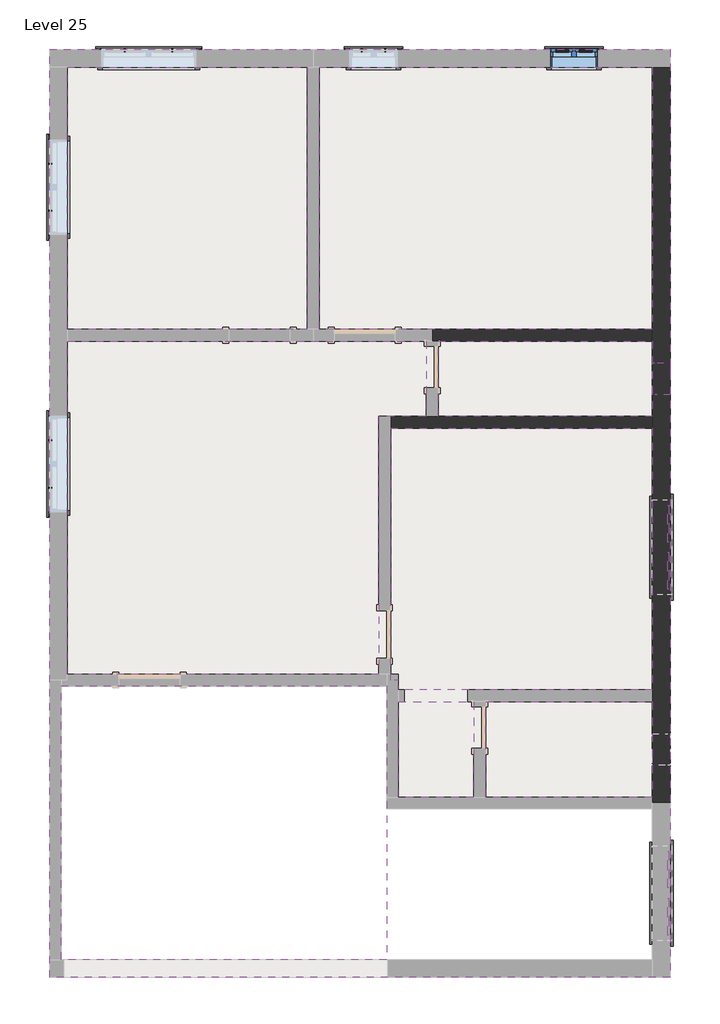
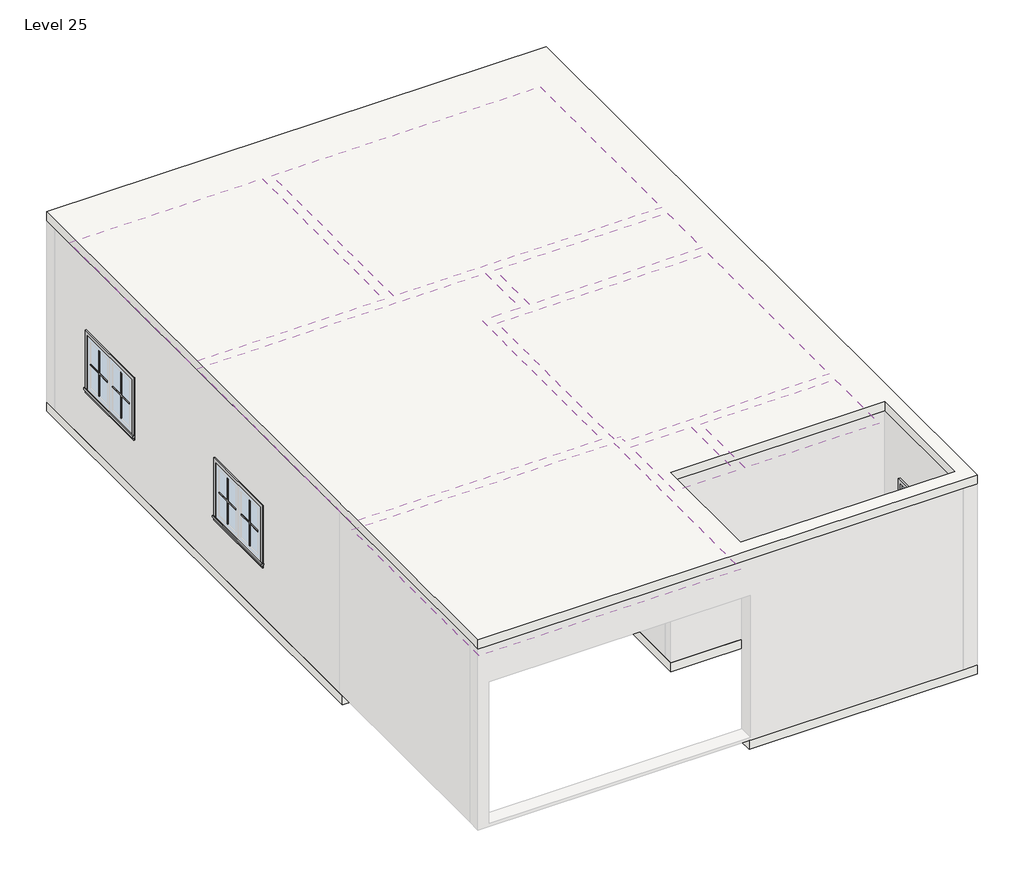
# One storey, part 2 of 2: 44 proxies, 8 coverings, 3 walls, 3 windows, 2 slabs.
"""IFC4 building model written with IfcOpenShell, lengths in millimetres."""

from ifc_helpers import new_model, si_unit, frame, origin, place, context, project, spatial, polyline, outline, extrude, faceted_brep, transform, mapped, element, save
from components import muntin_pattern_2x2_muntin_pattern_2x2_2357e71d, muntin_pattern_2x2_muntin_pattern_2x2_302d8f29, muntin_pattern_2x2_muntin_pattern_2x2_53152e2c, muntin_pattern_2x2_muntin_pattern_2x2_e8f3e573, trim_window_exterior_flat_with_sill_c4e67c73, trim_window_exterior_flat_with_sill_a665a915, trim_window_interior_flat_picture_frame_cf1733af, trim_window_interior_flat_picture_frame_d485c387, fixed_2_415b3208, window_casement_double_3_c417fced

model = new_model("IFC4")

# Units and contexts
model_context = context("Model", 3, world=origin())
ifc_project = project(units=[si_unit("LENGTHUNIT", "METRE", prefix="MILLI")], contexts=[model_context])

# Site, building, storey
site = spatial("IfcSite", under=ifc_project)
building = spatial("IfcBuilding", under=site)
storey = spatial("IfcBuildingStorey", under=building, Name="Level 25", Elevation=22402.8)

# Proxies
placement = place(None, origin())
muntin_pattern_2x2_muntin_pattern_2x2_shape = muntin_pattern_2x2_muntin_pattern_2x2_2357e71d(model_context)
element("IfcBuildingElementProxy", 1, Name="Muntin Pattern_2x2 : Muntin Pattern_2x2", ObjectType="Muntin Pattern_2x2 : Muntin Pattern_2x2", at=placement, inside=storey, context=model_context, shape_type="MappedRepresentation", body=[
    mapped(muntin_pattern_2x2_muntin_pattern_2x2_shape, transform((-4942.3279463, 5897.3080275, 23387.05), x_axis=(1.0, 0.0, 0.0), y_axis=(0.0, 1.0, 0.0), z_axis=(0.0, 0.0, 1.0))),
])
element("IfcBuildingElementProxy", 2, Name="Muntin Pattern_2x2 : Muntin Pattern_2x2", ObjectType="Muntin Pattern_2x2 : Muntin Pattern_2x2", at=placement, inside=storey, context=model_context, shape_type="MappedRepresentation", body=[
    mapped(muntin_pattern_2x2_muntin_pattern_2x2_shape, transform((-5899.5904463, 3838.3205275, 23387.05), x_axis=(0.0, 1.0, 0.0), y_axis=(-1.0, 0.0, 0.0), z_axis=(0.0, 0.0, 1.0))),
])
element("IfcBuildingElementProxy", 3, Name="Muntin Pattern_2x2 : Muntin Pattern_2x2", ObjectType="Muntin Pattern_2x2 : Muntin Pattern_2x2", at=placement, inside=storey, context=model_context, shape_type="MappedRepresentation", body=[
    mapped(muntin_pattern_2x2_muntin_pattern_2x2_shape, transform((-5899.5904463, 293.4330275, 23387.05), x_axis=(0.0, 1.0, 0.0), y_axis=(-1.0, 0.0, 0.0), z_axis=(0.0, 0.0, 1.0))),
])
element("IfcBuildingElementProxy", 4, Name="Muntin Pattern_2x2 : Muntin Pattern_2x2", ObjectType="Muntin Pattern_2x2 : Muntin Pattern_2x2", at=placement, inside=storey, context=model_context, shape_type="MappedRepresentation", body=[
    mapped(muntin_pattern_2x2_muntin_pattern_2x2_shape, transform((2031.5595537, -166.9419725, 23691.85), x_axis=(0.0, -1.0, 0.0), y_axis=(1.0, 0.0, 0.0), z_axis=(0.0, 0.0, 1.0))),
])
element("IfcBuildingElementProxy", 5, Name="Muntin Pattern_2x2 : Muntin Pattern_2x2", ObjectType="Muntin Pattern_2x2 : Muntin Pattern_2x2", at=placement, inside=storey, context=model_context, shape_type="MappedRepresentation", body=[
    mapped(muntin_pattern_2x2_muntin_pattern_2x2_shape, transform((2031.5595537, -4599.2419725, 23691.85), x_axis=(0.0, -1.0, 0.0), y_axis=(1.0, 0.0, 0.0), z_axis=(0.0, 0.0, 1.0))),
])
element("IfcBuildingElementProxy", 6, Name="Muntin Pattern_2x2 : Muntin Pattern_2x2", ObjectType="Muntin Pattern_2x2 : Muntin Pattern_2x2", at=placement, inside=storey, context=model_context, shape_type="MappedRepresentation", body=[
    mapped(muntin_pattern_2x2_muntin_pattern_2x2_shape, transform((-4942.3279463, 5897.3080275, 23387.05), x_axis=(1.0, 0.0, 0.0), y_axis=(0.0, 1.0, 0.0), z_axis=(0.0, 0.0, 1.0))),
])
element("IfcBuildingElementProxy", 7, Name="Muntin Pattern_2x2 : Muntin Pattern_2x2", ObjectType="Muntin Pattern_2x2 : Muntin Pattern_2x2", at=placement, inside=storey, context=model_context, shape_type="MappedRepresentation", body=[
    mapped(muntin_pattern_2x2_muntin_pattern_2x2_shape, transform((2031.5595537, -4599.2419725, 23691.85), x_axis=(0.0, -1.0, 0.0), y_axis=(1.0, 0.0, 0.0), z_axis=(0.0, 0.0, 1.0))),
])
muntin_pattern_2x2_muntin_pattern_2x2_2_shape = muntin_pattern_2x2_muntin_pattern_2x2_302d8f29(model_context)
element("IfcBuildingElementProxy", 8, Name="Muntin Pattern_2x2 : Muntin Pattern_2x2", ObjectType="Muntin Pattern_2x2 : Muntin Pattern_2x2", at=placement, inside=storey, context=model_context, shape_type="MappedRepresentation", body=[
    mapped(muntin_pattern_2x2_muntin_pattern_2x2_2_shape, transform((-4335.9029463, 5897.3080275, 23387.05), x_axis=(-1.0, 0.0, 0.0), y_axis=(0.0, -1.0, 0.0), z_axis=(0.0, 0.0, 1.0))),
])
element("IfcBuildingElementProxy", 9, Name="Muntin Pattern_2x2 : Muntin Pattern_2x2", ObjectType="Muntin Pattern_2x2 : Muntin Pattern_2x2", at=placement, inside=storey, context=model_context, shape_type="MappedRepresentation", body=[
    mapped(muntin_pattern_2x2_muntin_pattern_2x2_2_shape, transform((-5899.5904463, 4444.7455275, 23387.05), x_axis=(0.0, -1.0, 0.0), y_axis=(1.0, 0.0, 0.0), z_axis=(0.0, 0.0, 1.0))),
])
element("IfcBuildingElementProxy", 10, Name="Muntin Pattern_2x2 : Muntin Pattern_2x2", ObjectType="Muntin Pattern_2x2 : Muntin Pattern_2x2", at=placement, inside=storey, context=model_context, shape_type="MappedRepresentation", body=[
    mapped(muntin_pattern_2x2_muntin_pattern_2x2_2_shape, transform((-5899.5904463, 899.8580275, 23387.05), x_axis=(0.0, -1.0, 0.0), y_axis=(1.0, 0.0, 0.0), z_axis=(0.0, 0.0, 1.0))),
])
element("IfcBuildingElementProxy", 11, Name="Muntin Pattern_2x2 : Muntin Pattern_2x2", ObjectType="Muntin Pattern_2x2 : Muntin Pattern_2x2", at=placement, inside=storey, context=model_context, shape_type="MappedRepresentation", body=[
    mapped(muntin_pattern_2x2_muntin_pattern_2x2_2_shape, transform((2031.5595537, -773.3669725, 23691.85), x_axis=(0.0, 1.0, 0.0), y_axis=(-1.0, 0.0, 0.0), z_axis=(0.0, 0.0, 1.0))),
])
element("IfcBuildingElementProxy", 12, Name="Muntin Pattern_2x2 : Muntin Pattern_2x2", ObjectType="Muntin Pattern_2x2 : Muntin Pattern_2x2", at=placement, inside=storey, context=model_context, shape_type="MappedRepresentation", body=[
    mapped(muntin_pattern_2x2_muntin_pattern_2x2_2_shape, transform((2031.5595537, -5205.6669725, 23691.85), x_axis=(0.0, 1.0, 0.0), y_axis=(-1.0, 0.0, 0.0), z_axis=(0.0, 0.0, 1.0))),
])
element("IfcBuildingElementProxy", 13, Name="Muntin Pattern_2x2 : Muntin Pattern_2x2", ObjectType="Muntin Pattern_2x2 : Muntin Pattern_2x2", at=placement, inside=storey, context=model_context, shape_type="MappedRepresentation", body=[
    mapped(muntin_pattern_2x2_muntin_pattern_2x2_2_shape, transform((-4335.9029463, 5897.3080275, 23387.05), x_axis=(-1.0, 0.0, 0.0), y_axis=(0.0, -1.0, 0.0), z_axis=(0.0, 0.0, 1.0))),
])
element("IfcBuildingElementProxy", 14, Name="Muntin Pattern_2x2 : Muntin Pattern_2x2", ObjectType="Muntin Pattern_2x2 : Muntin Pattern_2x2", at=placement, inside=storey, context=model_context, shape_type="MappedRepresentation", body=[
    mapped(muntin_pattern_2x2_muntin_pattern_2x2_2_shape, transform((2031.5595537, -5205.6669725, 23691.85), x_axis=(0.0, 1.0, 0.0), y_axis=(-1.0, 0.0, 0.0), z_axis=(0.0, 0.0, 1.0))),
])
muntin_pattern_2x2_muntin_pattern_2x2_3_shape = muntin_pattern_2x2_muntin_pattern_2x2_53152e2c(model_context)
element("IfcBuildingElementProxy", 15, Name="Muntin Pattern_2x2 : Muntin Pattern_2x2", ObjectType="Muntin Pattern_2x2 : Muntin Pattern_2x2", at=placement, inside=storey, context=model_context, shape_type="MappedRepresentation", body=[
    mapped(muntin_pattern_2x2_muntin_pattern_2x2_3_shape, transform((-1907.0279463, 5897.3080275, 23387.05), x_axis=(1.0, 0.0, 0.0), y_axis=(0.0, 1.0, 0.0), z_axis=(0.0, 0.0, 1.0))),
])
element("IfcBuildingElementProxy", 16, Name="Muntin Pattern_2x2 : Muntin Pattern_2x2", ObjectType="Muntin Pattern_2x2 : Muntin Pattern_2x2", at=placement, inside=storey, context=model_context, shape_type="MappedRepresentation", body=[
    mapped(muntin_pattern_2x2_muntin_pattern_2x2_3_shape, transform((658.3720537, 5897.3080275, 23387.05), x_axis=(1.0, 0.0, 0.0), y_axis=(0.0, 1.0, 0.0), z_axis=(0.0, 0.0, 1.0))),
])
element("IfcBuildingElementProxy", 17, Name="Muntin Pattern_2x2 : Muntin Pattern_2x2", ObjectType="Muntin Pattern_2x2 : Muntin Pattern_2x2", at=placement, inside=storey, context=model_context, shape_type="MappedRepresentation", body=[
    mapped(muntin_pattern_2x2_muntin_pattern_2x2_3_shape, transform((-1907.0279463, 5897.3080275, 23387.05), x_axis=(1.0, 0.0, 0.0), y_axis=(0.0, 1.0, 0.0), z_axis=(0.0, 0.0, 1.0))),
])
element("IfcBuildingElementProxy", 18, Name="Muntin Pattern_2x2 : Muntin Pattern_2x2", ObjectType="Muntin Pattern_2x2 : Muntin Pattern_2x2", at=placement, inside=storey, context=model_context, shape_type="MappedRepresentation", body=[
    mapped(muntin_pattern_2x2_muntin_pattern_2x2_3_shape, transform((658.3720537, 5897.3080275, 23387.05), x_axis=(1.0, 0.0, 0.0), y_axis=(0.0, 1.0, 0.0), z_axis=(0.0, 0.0, 1.0))),
])
muntin_pattern_2x2_muntin_pattern_2x2_4_shape = muntin_pattern_2x2_muntin_pattern_2x2_e8f3e573(model_context)
element("IfcBuildingElementProxy", 19, Name="Muntin Pattern_2x2 : Muntin Pattern_2x2", ObjectType="Muntin Pattern_2x2 : Muntin Pattern_2x2", at=placement, inside=storey, context=model_context, shape_type="MappedRepresentation", body=[
    mapped(muntin_pattern_2x2_muntin_pattern_2x2_4_shape, transform((-1605.4029463, 5897.3080275, 23387.05), x_axis=(-1.0, 0.0, 0.0), y_axis=(0.0, -1.0, 0.0), z_axis=(0.0, 0.0, 1.0))),
])
element("IfcBuildingElementProxy", 20, Name="Muntin Pattern_2x2 : Muntin Pattern_2x2", ObjectType="Muntin Pattern_2x2 : Muntin Pattern_2x2", at=placement, inside=storey, context=model_context, shape_type="MappedRepresentation", body=[
    mapped(muntin_pattern_2x2_muntin_pattern_2x2_4_shape, transform((959.9970537, 5897.3080275, 23387.05), x_axis=(-1.0, 0.0, 0.0), y_axis=(0.0, -1.0, 0.0), z_axis=(0.0, 0.0, 1.0))),
])
element("IfcBuildingElementProxy", 21, Name="Muntin Pattern_2x2 : Muntin Pattern_2x2", ObjectType="Muntin Pattern_2x2 : Muntin Pattern_2x2", at=placement, inside=storey, context=model_context, shape_type="MappedRepresentation", body=[
    mapped(muntin_pattern_2x2_muntin_pattern_2x2_4_shape, transform((-1605.4029463, 5897.3080275, 23387.05), x_axis=(-1.0, 0.0, 0.0), y_axis=(0.0, -1.0, 0.0), z_axis=(0.0, 0.0, 1.0))),
])
element("IfcBuildingElementProxy", 22, Name="Muntin Pattern_2x2 : Muntin Pattern_2x2", ObjectType="Muntin Pattern_2x2 : Muntin Pattern_2x2", at=placement, inside=storey, context=model_context, shape_type="MappedRepresentation", body=[
    mapped(muntin_pattern_2x2_muntin_pattern_2x2_4_shape, transform((959.9970537, 5897.3080275, 23387.05), x_axis=(-1.0, 0.0, 0.0), y_axis=(0.0, -1.0, 0.0), z_axis=(0.0, 0.0, 1.0))),
])
trim_window_exterior_flat_with_sill_shape = trim_window_exterior_flat_with_sill_c4e67c73(model_context)
element("IfcBuildingElementProxy", 23, Name="Trim-Window-Exterior-Flat : with Sill", ObjectType="Trim-Window-Exterior-Flat : with Sill", at=placement, inside=storey, context=model_context, shape_type="MappedRepresentation", body=[
    mapped(trim_window_exterior_flat_with_sill_shape, transform((-4639.1154463, 5906.8330275, 24231.6), x_axis=(-1.0, 0.0, 0.0), y_axis=(0.0, 0.0, 1.0), z_axis=(0.0, 1.0, 0.0))),
])
element("IfcBuildingElementProxy", 24, Name="Trim-Window-Exterior-Flat : with Sill", ObjectType="Trim-Window-Exterior-Flat : with Sill", at=placement, inside=storey, context=model_context, shape_type="MappedRepresentation", body=[
    mapped(trim_window_exterior_flat_with_sill_shape, transform((-5909.1154463, 4141.5330275, 24231.6), x_axis=(0.0, -1.0, 0.0), y_axis=(0.0, 0.0, 1.0), z_axis=(-1.0, 0.0, 0.0))),
])
element("IfcBuildingElementProxy", 25, Name="Trim-Window-Exterior-Flat : with Sill", ObjectType="Trim-Window-Exterior-Flat : with Sill", at=placement, inside=storey, context=model_context, shape_type="MappedRepresentation", body=[
    mapped(trim_window_exterior_flat_with_sill_shape, transform((-5909.1154463, 596.6455275, 24231.6), x_axis=(0.0, -1.0, 0.0), y_axis=(0.0, 0.0, 1.0), z_axis=(-1.0, 0.0, 0.0))),
])
element("IfcBuildingElementProxy", 26, Name="Trim-Window-Exterior-Flat : with Sill", ObjectType="Trim-Window-Exterior-Flat : with Sill", at=placement, inside=storey, context=model_context, shape_type="MappedRepresentation", body=[
    mapped(trim_window_exterior_flat_with_sill_shape, transform((2041.0845537, -470.1544725, 24536.4), x_axis=(0.0, 1.0, 0.0), y_axis=(0.0, 0.0, 1.0), z_axis=(1.0, 0.0, 0.0))),
])
element("IfcBuildingElementProxy", 27, Name="Trim-Window-Exterior-Flat : with Sill", ObjectType="Trim-Window-Exterior-Flat : with Sill", at=placement, inside=storey, context=model_context, shape_type="MappedRepresentation", body=[
    mapped(trim_window_exterior_flat_with_sill_shape, transform((2041.0845537, -4902.4544725, 24536.4), x_axis=(0.0, 1.0, 0.0), y_axis=(0.0, 0.0, 1.0), z_axis=(1.0, 0.0, 0.0))),
])
element("IfcBuildingElementProxy", 28, Name="Trim-Window-Exterior-Flat : with Sill", ObjectType="Trim-Window-Exterior-Flat : with Sill", at=placement, inside=storey, context=model_context, shape_type="MappedRepresentation", body=[
    mapped(trim_window_exterior_flat_with_sill_shape, transform((-4639.1154463, 5906.8330275, 24231.6), x_axis=(-1.0, 0.0, 0.0), y_axis=(0.0, 0.0, 1.0), z_axis=(0.0, 1.0, 0.0))),
])
element("IfcBuildingElementProxy", 29, Name="Trim-Window-Exterior-Flat : with Sill", ObjectType="Trim-Window-Exterior-Flat : with Sill", at=placement, inside=storey, context=model_context, shape_type="MappedRepresentation", body=[
    mapped(trim_window_exterior_flat_with_sill_shape, transform((2041.0845537, -4902.4544725, 24536.4), x_axis=(0.0, 1.0, 0.0), y_axis=(0.0, 0.0, 1.0), z_axis=(1.0, 0.0, 0.0))),
])
trim_window_exterior_flat_with_sill_2_shape = trim_window_exterior_flat_with_sill_a665a915(model_context)
element("IfcBuildingElementProxy", 30, Name="Trim-Window-Exterior-Flat : with Sill", ObjectType="Trim-Window-Exterior-Flat : with Sill", at=placement, inside=storey, context=model_context, shape_type="MappedRepresentation", body=[
    mapped(trim_window_exterior_flat_with_sill_2_shape, transform((-1756.2154463, 5906.8330275, 24231.6), x_axis=(-1.0, 0.0, 0.0), y_axis=(0.0, 0.0, 1.0), z_axis=(0.0, 1.0, 0.0))),
])
element("IfcBuildingElementProxy", 31, Name="Trim-Window-Exterior-Flat : with Sill", ObjectType="Trim-Window-Exterior-Flat : with Sill", at=placement, inside=storey, context=model_context, shape_type="MappedRepresentation", body=[
    mapped(trim_window_exterior_flat_with_sill_2_shape, transform((809.1845537, 5906.8330275, 24231.6), x_axis=(-1.0, 0.0, 0.0), y_axis=(0.0, 0.0, 1.0), z_axis=(0.0, 1.0, 0.0))),
])
element("IfcBuildingElementProxy", 32, Name="Trim-Window-Exterior-Flat : with Sill", ObjectType="Trim-Window-Exterior-Flat : with Sill", at=placement, inside=storey, context=model_context, shape_type="MappedRepresentation", body=[
    mapped(trim_window_exterior_flat_with_sill_2_shape, transform((-1756.2154463, 5906.8330275, 24231.6), x_axis=(-1.0, 0.0, 0.0), y_axis=(0.0, 0.0, 1.0), z_axis=(0.0, 1.0, 0.0))),
])
element("IfcBuildingElementProxy", 33, Name="Trim-Window-Exterior-Flat : with Sill", ObjectType="Trim-Window-Exterior-Flat : with Sill", at=placement, inside=storey, context=model_context, shape_type="MappedRepresentation", body=[
    mapped(trim_window_exterior_flat_with_sill_2_shape, transform((809.1845537, 5906.8330275, 24231.6), x_axis=(-1.0, 0.0, 0.0), y_axis=(0.0, 0.0, 1.0), z_axis=(0.0, 1.0, 0.0))),
])
trim_window_interior_flat_picture_frame_shape = trim_window_interior_flat_picture_frame_cf1733af(model_context)
element("IfcBuildingElementProxy", 34, Name="Trim-Window-Interior-Flat : Picture Frame", ObjectType="Trim-Window-Interior-Flat : Picture Frame", at=placement, inside=storey, context=model_context, shape_type="MappedRepresentation", body=[
    mapped(trim_window_interior_flat_picture_frame_shape, transform((-4639.1154463, 5678.2330275, 24231.6), x_axis=(1.0, 0.0, 0.0), y_axis=(0.0, 0.0, 1.0), z_axis=(0.0, -1.0, 0.0))),
])
element("IfcBuildingElementProxy", 35, Name="Trim-Window-Interior-Flat : Picture Frame", ObjectType="Trim-Window-Interior-Flat : Picture Frame", at=placement, inside=storey, context=model_context, shape_type="MappedRepresentation", body=[
    mapped(trim_window_interior_flat_picture_frame_shape, transform((-5680.5154463, 4141.5330275, 24231.6), x_axis=(0.0, 1.0, 0.0), y_axis=(0.0, 0.0, 1.0), z_axis=(1.0, 0.0, 0.0))),
])
element("IfcBuildingElementProxy", 36, Name="Trim-Window-Interior-Flat : Picture Frame", ObjectType="Trim-Window-Interior-Flat : Picture Frame", at=placement, inside=storey, context=model_context, shape_type="MappedRepresentation", body=[
    mapped(trim_window_interior_flat_picture_frame_shape, transform((-5680.5154463, 596.6455275, 24231.6), x_axis=(0.0, 1.0, 0.0), y_axis=(0.0, 0.0, 1.0), z_axis=(1.0, 0.0, 0.0))),
])
element("IfcBuildingElementProxy", 37, Name="Trim-Window-Interior-Flat : Picture Frame", ObjectType="Trim-Window-Interior-Flat : Picture Frame", at=placement, inside=storey, context=model_context, shape_type="MappedRepresentation", body=[
    mapped(trim_window_interior_flat_picture_frame_shape, transform((1812.4845537, -470.1544725, 24536.4), x_axis=(0.0, -1.0, 0.0), y_axis=(0.0, 0.0, 1.0), z_axis=(-1.0, 0.0, 0.0))),
])
element("IfcBuildingElementProxy", 38, Name="Trim-Window-Interior-Flat : Picture Frame", ObjectType="Trim-Window-Interior-Flat : Picture Frame", at=placement, inside=storey, context=model_context, shape_type="MappedRepresentation", body=[
    mapped(trim_window_interior_flat_picture_frame_shape, transform((1812.4845537, -4902.4544725, 24536.4), x_axis=(0.0, -1.0, 0.0), y_axis=(0.0, 0.0, 1.0), z_axis=(-1.0, 0.0, 0.0))),
])
element("IfcBuildingElementProxy", 39, Name="Trim-Window-Interior-Flat : Picture Frame", ObjectType="Trim-Window-Interior-Flat : Picture Frame", at=placement, inside=storey, context=model_context, shape_type="MappedRepresentation", body=[
    mapped(trim_window_interior_flat_picture_frame_shape, transform((-4639.1154463, 5678.2330275, 24231.6), x_axis=(1.0, 0.0, 0.0), y_axis=(0.0, 0.0, 1.0), z_axis=(0.0, -1.0, 0.0))),
])
element("IfcBuildingElementProxy", 40, Name="Trim-Window-Interior-Flat : Picture Frame", ObjectType="Trim-Window-Interior-Flat : Picture Frame", at=placement, inside=storey, context=model_context, shape_type="MappedRepresentation", body=[
    mapped(trim_window_interior_flat_picture_frame_shape, transform((1812.4845537, -4902.4544725, 24536.4), x_axis=(0.0, -1.0, 0.0), y_axis=(0.0, 0.0, 1.0), z_axis=(-1.0, 0.0, 0.0))),
])
trim_window_interior_flat_picture_frame_2_shape = trim_window_interior_flat_picture_frame_d485c387(model_context)
element("IfcBuildingElementProxy", 41, Name="Trim-Window-Interior-Flat : Picture Frame", ObjectType="Trim-Window-Interior-Flat : Picture Frame", at=placement, inside=storey, context=model_context, shape_type="MappedRepresentation", body=[
    mapped(trim_window_interior_flat_picture_frame_2_shape, transform((-1756.2154463, 5678.2330275, 24231.6), x_axis=(1.0, 0.0, 0.0), y_axis=(0.0, 0.0, 1.0), z_axis=(0.0, -1.0, 0.0))),
])
element("IfcBuildingElementProxy", 42, Name="Trim-Window-Interior-Flat : Picture Frame", ObjectType="Trim-Window-Interior-Flat : Picture Frame", at=placement, inside=storey, context=model_context, shape_type="MappedRepresentation", body=[
    mapped(trim_window_interior_flat_picture_frame_2_shape, transform((809.1845537, 5678.2330275, 24231.6), x_axis=(1.0, 0.0, 0.0), y_axis=(0.0, 0.0, 1.0), z_axis=(0.0, -1.0, 0.0))),
])
element("IfcBuildingElementProxy", 43, Name="Trim-Window-Interior-Flat : Picture Frame", ObjectType="Trim-Window-Interior-Flat : Picture Frame", at=placement, inside=storey, context=model_context, shape_type="MappedRepresentation", body=[
    mapped(trim_window_interior_flat_picture_frame_2_shape, transform((-1756.2154463, 5678.2330275, 24231.6), x_axis=(1.0, 0.0, 0.0), y_axis=(0.0, 0.0, 1.0), z_axis=(0.0, -1.0, 0.0))),
])
element("IfcBuildingElementProxy", 44, Name="Trim-Window-Interior-Flat : Picture Frame", ObjectType="Trim-Window-Interior-Flat : Picture Frame", at=placement, inside=storey, context=model_context, shape_type="MappedRepresentation", body=[
    mapped(trim_window_interior_flat_picture_frame_2_shape, transform((809.1845537, 5678.2330275, 24231.6), x_axis=(1.0, 0.0, 0.0), y_axis=(0.0, 0.0, 1.0), z_axis=(0.0, -1.0, 0.0))),
])

# Coverings
element("IfcCovering", 45, ObjectType="2' x 4' ACT System", at=placement, inside=storey, context=model_context, shape_type="SweptSolid", body=[
    extrude(outline(polyline([(-5680.5154463, 2323.8455275), (-5680.5154463, 5678.2330275), (-2607.1154463, 5678.2330275), (-2607.1154463, 2323.8455275), (-5680.5154463, 2323.8455275)])), frame((0.0, 0.0, 25146.0), z_axis=(0.0, 0.0, 1.0), x_axis=(1.0, 0.0, 0.0)), (0.0, 0.0, 1.0), 57.15),
])
element("IfcCovering", 46, ObjectType="2' x 4' ACT System", at=placement, inside=storey, context=model_context, shape_type="SweptSolid", body=[
    extrude(outline(polyline([(-2454.7154463, 2323.8455275), (-2454.7154463, 5678.2330275), (1812.4845537, 5678.2330275), (1812.4845537, 2323.8455275), (-2454.7154463, 2323.8455275)])), frame((0.0, 0.0, 25146.0), z_axis=(0.0, 0.0, 1.0), x_axis=(1.0, 0.0, 0.0)), (0.0, 0.0, 1.0), 57.15),
])
element("IfcCovering", 47, ObjectType="2' x 4' ACT System", at=placement, inside=storey, context=model_context, shape_type="SweptSolid", body=[
    extrude(outline(polyline([(-5680.5154463, -2095.7544725), (-5680.5154463, 2171.4455275), (-1083.1154463, 2171.4455275), (-1083.1154463, 1206.2455275), (-1692.7154463, 1206.2455275), (-1692.7154463, -2095.7544725), (-5680.5154463, -2095.7544725)])), frame((0.0, 0.0, 25146.0), z_axis=(0.0, 0.0, 1.0), x_axis=(1.0, 0.0, 0.0)), (0.0, 0.0, 1.0), 57.15),
])
element("IfcCovering", 48, ObjectType="2' x 4' ACT System", at=placement, inside=storey, context=model_context, shape_type="SweptSolid", body=[
    extrude(outline(polyline([(-930.7154463, 2171.4455275), (1812.4845537, 2171.4455275), (1812.4845537, 1206.2455275), (-930.7154463, 1206.2455275), (-930.7154463, 2171.4455275)])), frame((0.0, 0.0, 25146.0), z_axis=(0.0, 0.0, 1.0), x_axis=(1.0, 0.0, 0.0)), (0.0, 0.0, 1.0), 57.15),
])
element("IfcCovering", 49, ObjectType="2' x 4' ACT System", at=placement, inside=storey, context=model_context, shape_type="SweptSolid", body=[
    extrude(outline(polyline([(1812.4845537, 1053.8455275), (1812.4845537, -2298.9544725), (-1438.7154463, -2298.9544725), (-1438.7154463, -2171.9544725), (-1540.3154463, -2171.9544725), (-1540.3154463, 1053.8455275), (1812.4845537, 1053.8455275)])), frame((0.0, 0.0, 25146.0), z_axis=(0.0, 0.0, 1.0), x_axis=(1.0, 0.0, 0.0)), (0.0, 0.0, 1.0), 57.15),
])
element("IfcCovering", 50, ObjectType="2' x 4' ACT System", at=placement, inside=storey, context=model_context, shape_type="SweptSolid", body=[
    extrude(outline(polyline([(1812.4845537, -2451.3544725), (1812.4845537, -3670.5544725), (-321.1154463, -3670.5544725), (-321.1154463, -2451.3544725), (1812.4845537, -2451.3544725)])), frame((0.0, 0.0, 25146.0), z_axis=(0.0, 0.0, 1.0), x_axis=(1.0, 0.0, 0.0)), (0.0, 0.0, 1.0), 57.15),
])
element("IfcCovering", 51, ObjectType="2' x 4' ACT System", at=placement, inside=storey, context=model_context, shape_type="SweptSolid", body=[
    extrude(outline(polyline([(-473.5154463, -2451.3544725), (-473.5154463, -3670.5544725), (-1438.7154463, -3670.5544725), (-1438.7154463, -2451.3544725), (-473.5154463, -2451.3544725)])), frame((0.0, 0.0, 25146.0), z_axis=(0.0, 0.0, 1.0), x_axis=(1.0, 0.0, 0.0)), (0.0, 0.0, 1.0), 57.15),
])
element("IfcCovering", 52, ObjectType="2' x 4' ACT System", at=placement, inside=storey, context=model_context, shape_type="SweptSolid", body=[
    extrude(outline(polyline([(-1591.1154463, -2248.1544725), (-1591.1154463, -5753.3544725), (-5756.7154463, -5753.3544725), (-5756.7154463, -2248.1544725), (-1591.1154463, -2248.1544725)])), frame((0.0, 0.0, 25146.0), z_axis=(0.0, 0.0, 1.0), x_axis=(1.0, 0.0, 0.0)), (0.0, 0.0, 1.0), 57.15),
])

# Slabs
element("IfcSlab", 53, ObjectType="Generic - 6\"", at=placement, inside=storey, context=model_context, shape_type="SweptSolid", body=[
    extrude(outline(polyline([(-5909.1154463, -2248.1544725), (-5909.1154463, 5906.8330275), (2041.0845537, 5906.8330275), (2041.0845537, -5981.9544725), (-1591.1154463, -5981.9544725), (-1591.1154463, -5753.3544725), (1812.4845537, -5753.3544725), (1812.4845537, -3822.9544725), (-1591.1154463, -3822.9544725), (-1591.1154463, -2248.1544725), (-5756.7154463, -2248.1544725), (-5909.1154463, -2248.1544725)])), frame((0.0, 0.0, 22250.4), z_axis=(0.0, 0.0, 1.0), x_axis=(1.0, 0.0, 0.0)), (0.0, 0.0, 1.0), 152.4),
])
element("IfcSlab", 54, ObjectType="Generic - 6\"", at=placement, inside=storey, context=model_context, shape_type="SweptSolid", body=[
    extrude(outline(polyline([(2041.0845537, 5906.8330275), (2041.0845537, -5981.9544725), (-5909.1154463, -5981.9544725), (-5909.1154463, 5906.8330275), (2041.0845537, 5906.8330275)]), holes=[polyline([(1812.4845537, -3822.9544725), (-1591.1154463, -3822.9544725), (-1591.1154463, -5753.3544725), (1812.4845537, -5753.3544725), (1812.4845537, -3822.9544725)])]), frame((0.0, 0.0, 25450.8), z_axis=(0.0, 0.0, 1.0), x_axis=(1.0, 0.0, 0.0)), (0.0, 0.0, 1.0), 152.4),
])

# Walls
element("IfcWall", 55, ObjectType="Generic - 6\"", at=placement, inside=storey, context=model_context, shape_type="Brep", body=[
    faceted_brep([(-1540.3154463, 1053.8455275, 22402.8), (1812.4845537, 1053.8455275, 22402.8), (1812.4845537, 1053.8455275, 25450.8), (-1540.3154463, 1053.8455275, 25450.8), (-1540.3154463, 1206.2455275, 22402.8), (-1540.3154463, 1206.2455275, 25450.8), (-1083.1154463, 1206.2455275, 25450.8), (-930.7154463, 1206.2455275, 25450.8), (1812.4845537, 1206.2455275, 25450.8), (1812.4845537, 1206.2455275, 22402.8), (-930.7154463, 1206.2455275, 22402.8), (-1083.1154463, 1206.2455275, 22402.8)], [[[0, 1, 2, 3]], [[4, 5, 6, 7, 8, 9, 10, 11]], [[1, 0, 4, 11, 10, 9]], [[3, 2, 8, 7, 6, 5]], [[0, 3, 5, 4]], [[2, 1, 9, 8]]]),
])
element("IfcWall", 56, ObjectType="Generic - 6\"", at=placement, inside=storey, context=model_context, shape_type="Brep", body=[
    faceted_brep([(1812.4845537, 2323.8455275, 22402.8), (-1006.9154463, 2323.8455275, 22402.8), (-1006.9154463, 2323.8455275, 25450.8), (1812.4845537, 2323.8455275, 25450.8), (1812.4845537, 2171.4455275, 22402.8), (1812.4845537, 2171.4455275, 25450.8), (-930.7154463, 2171.4455275, 25450.8), (-1006.9154463, 2171.4455275, 25450.8), (-1006.9154463, 2171.4455275, 22402.8), (-930.7154463, 2171.4455275, 22402.8)], [[[0, 1, 2, 3]], [[4, 5, 6, 7, 8, 9]], [[1, 0, 4, 9, 8]], [[2, 1, 8, 7]], [[3, 2, 7, 6, 5]], [[0, 3, 5, 4]]]),
])
element("IfcWall", 57, ObjectType="Generic - 9\"", at=placement, inside=storey, context=model_context, shape_type="Brep", body=[
    faceted_brep([(1812.4845537, 5678.2330275, 22402.8), (1812.4845537, 2323.8455275, 22402.8), (1812.4845537, 2171.4455275, 22402.8), (1812.4845537, 1206.2455275, 22402.8), (1812.4845537, 1053.8455275, 22402.8), (1812.4845537, -2298.9544725, 22402.8), (1812.4845537, -2451.3544725, 22402.8), (1812.4845537, -3670.5544725, 22402.8), (1812.4845537, -3746.7544725, 22402.8), (1812.4845537, -3746.7544725, 25450.8), (1812.4845537, -3670.5544725, 25450.8), (1812.4845537, -2451.3544725, 25450.8), (1812.4845537, -2298.9544725, 25450.8), (1812.4845537, 1053.8455275, 25450.8), (1812.4845537, 1206.2455275, 25450.8), (1812.4845537, 2171.4455275, 25450.8), (1812.4845537, 2323.8455275, 25450.8), (1812.4845537, 5678.2330275, 25450.8), (1812.4845537, -1079.7544725, 24536.4), (1812.4845537, -1079.7544725, 23622.0), (1812.4845537, 139.4455275, 23622.0), (1812.4845537, 139.4455275, 24536.4), (1812.4845537, -3264.1544725, 24841.2), (1812.4845537, -3264.1544725, 24231.6), (1812.4845537, -2857.7544725, 24231.6), (1812.4845537, -2857.7544725, 24841.2), (1812.4845537, 1892.0455275, 24841.2), (1812.4845537, 1485.6455275, 24841.2), (1812.4845537, 1485.6455275, 24231.6), (1812.4845537, 1892.0455275, 24231.6), (2041.0845537, 5678.2330275, 22402.8), (2041.0845537, 5678.2330275, 25450.8), (2041.0845537, -3746.7544725, 25450.8), (2041.0845537, -3746.7544725, 22402.8), (2041.0845537, -1079.7544725, 24536.4), (2041.0845537, 139.4455275, 24536.4), (2041.0845537, 139.4455275, 23622.0), (2041.0845537, -1079.7544725, 23622.0), (2041.0845537, -3264.1544725, 24841.2), (2041.0845537, -2857.7544725, 24841.2), (2041.0845537, -2857.7544725, 24231.6), (2041.0845537, -3264.1544725, 24231.6), (2041.0845537, 1892.0455275, 24841.2), (2041.0845537, 1892.0455275, 24231.6), (2041.0845537, 1485.6455275, 24231.6), (2041.0845537, 1485.6455275, 24841.2)], [[[0, 1, 2, 3, 4, 5, 6, 7, 8, 9, 10, 11, 12, 13, 14, 15, 16, 17], [18, 19, 20, 21], [22, 23, 24, 25], [26, 27, 28, 29]], [[30, 31, 32, 33], [34, 35, 36, 37], [38, 39, 40, 41], [42, 43, 44, 45]], [[8, 7, 6, 5, 4, 3, 2, 1, 0, 30, 33]], [[9, 8, 33, 32]], [[17, 16, 15, 14, 13, 12, 11, 10, 9, 32, 31]], [[0, 17, 31, 30]], [[19, 18, 34, 37]], [[20, 19, 37, 36]], [[21, 20, 36, 35]], [[18, 21, 35, 34]], [[23, 22, 38, 41]], [[24, 23, 41, 40]], [[25, 24, 40, 39]], [[22, 25, 39, 38]], [[43, 42, 26, 29]], [[44, 43, 29, 28]], [[45, 44, 28, 27]], [[42, 45, 27, 26]]]),
])

# Windows
fixed_2_shape = fixed_2_415b3208(model_context)
element("IfcWindow", 58, ObjectType="Fixed : 2'", at=placement, inside=storey, context=model_context, shape_type="MappedRepresentation", body=[
    mapped(fixed_2_shape, transform((1926.7845537, 1726.9455275, 23926.8), x_axis=(0.0, 1.0, 0.0), y_axis=(-1.0, 0.0, 0.0), z_axis=(0.0, 0.0, 1.0))),
])
window_casement_double_3_shape = window_casement_double_3_c417fced(model_context)
element("IfcWindow", 59, ObjectType="Window-Casement-Double : 3'", at=placement, inside=storey, context=model_context, shape_type="MappedRepresentation", body=[
    mapped(window_casement_double_3_shape, transform((809.1845537, 5792.5330275, 22402.8), x_axis=(1.0, 0.0, 0.0), y_axis=(0.0, 1.0, 0.0), z_axis=(0.0, 0.0, 1.0))),
])
element("IfcWindow", 60, ObjectType="Window-Casement-Double : 3'", at=placement, inside=storey, context=model_context, shape_type="MappedRepresentation", body=[
    mapped(window_casement_double_3_shape, transform((809.1845537, 5792.5330275, 22402.8), x_axis=(1.0, 0.0, 0.0), y_axis=(0.0, 1.0, 0.0), z_axis=(0.0, 0.0, 1.0))),
])

save(model, "model.ifc")

# Revit data of these elements
# Type "Muntin Pattern_2x2 : Muntin Pattern_2x2"
#   Width [instance default] = 4' - 0"
#   Thickness = 0' - 0 1/2"
#   Height [instance default] = 4' - 0"
#   Distance = 0' - 0 3/4"
#   Interior Material [instance default] = none
#   Exterior Material [instance default] = none
#   Default Elevation = 0
# Type "Trim-Window-Exterior-Flat : with Sill"
#   Trim Width = 0' - 2 1/4"
#   Trim Thickness_Picture Frame = 0' - 1 1/4"
#   Trim Thickness_with Sill = 0' - 0 3/4"
#   Sill Thickness = 0' - 1 1/4"
#   Opening Width [instance default] = 2' - 0"
#   Opening Height [instance default] = 3' - 0"
#   Default Elevation = 4' - 0"
#   Sill = yes
#   Picture Frame = no
#   Trim Material [instance default] = none
# Type "Trim-Window-Interior-Flat : Picture Frame"
#   Trim Thickness_Picture Frame = 0' - 1 1/4"
#   Trim Width = 0' - 2 1/4"
#   Trim Thickness_with Sill = 0' - 0 3/4"
#   Sill Thickness = 0' - 1 1/4"
#   Opening Width [instance default] = 2' - 0"
#   Opening Height [instance default] = 3' - 0"
#   Default Elevation = 4' - 0"
#   Sill = no
#   Picture Frame = yes
#   Trim Material [instance default] = none
# Type "2' x 4' ACT System"
#   Assembly Code = "C3030210"
#   built-in parameter 1002203 = 1 (stored number, unit not read)
#   built-in parameter 1002202 = 1 (stored number, unit not read)
#   Layers, outside or top first: 0' - 1 5/8" "Default" (function 1); 0' - 0 5/8" "Acoustic Ceiling Tile 24 x 48" (function 5)
# Type "Generic - 6\""
#   Assembly Code = "B1010"
#   Function = 0
#   Layers, outside or top first: 0' - 6" no material (function 1)
# Type "Generic - 6\""
#   Assembly Code = "B2010"
#   Layers, outside or top first: 0' - 6" no material (function 1)
# Type "Generic - 9\""
#   Assembly Code = "B2010"
#   Layers, outside or top first: 0' - 9" no material (function 1)
# Type "Fixed : 2'"
#   Type Mark = "20"
#   Construction Type Id = "GSP4R"
#   Assembly Code = "B2020100"
#   Analytic Construction = "1/8 in Pilkington single glazing"
#   Visual Light Transmittance = 0.9
#   Solar Heat Gain Coefficient = 0.78
#   Heat Transfer Coefficient (U) = 0.6496 BTU/(h·ft²·°F)
#   Height = 2' - 0"
#   Default Sill Height = 1' - 0"
#   Width = 1' - 4"
#   Window Inset = 0' - 0 3/4"
#   Define Thermal Properties by = 1
#   Glass Pane Material = Glass
#   Sash Material = Sash
#   Wall Closure = (empty or 0)
# Type "Window-Casement-Double : 3'"
#   Type Mark = "19"
#   Fire Rating = "0.5h"
#   Assembly Code = "B2020100"
#   Analytic Construction = "Double glazing - domestic"
#   Frame Extension [instance default] = 0' - 0 1/4"
#   Window Inset [instance default] = 0' - 0"
#   Wall Thickness [instance default] = 0' - 6"
#   Interior Wall Closure [instance default] = 0' - 2 1/4"
#   Half Width = 1' - 0"
#   Visual Light Transmittance = 0.81
#   Thermal Resistance (R) = 1.8146 (h·ft²·°F)/BTU
#   Solar Heat Gain Coefficient = 0.76
#   Rough Width = 2' - 0 1/2"
#   Rough Height = 3' - 0 1/2"
#   Height = 3' - 0"
#   Heat Transfer Coefficient (U) = 0.5511 BTU/(h·ft²·°F)
#   Exterior Wall Closure [instance default] = 0' - 1 1/4"
#   Extension Jamb [instance default] = 0' - 2 1/4"
#   Default Sill Height = 3' - 0"
#   Width = 2' - 0"
#   Muntin Visibility = yes
#   Interior Trim Visibility [instance default] = yes
#   Exterior Trim Visibility [instance default] = yes
#   Extension Jamb Visibility [instance default] = yes
#   Interior Trim Material = Wood - Stained
#   Muntin Pattern = Muntin Pattern_2x2 : Muntin Pattern_2x2
#   Interior Trim = Trim-Window-Interior-Flat : Picture Frame
#   Interior Frame Material = Wood - Stained
#   Glass Panel Material = Glass
#   Exterior Trim Material = Clad - White
#   Exterior Trim = Trim-Window-Exterior-Flat : with Sill
#   Exterior Frame Material = Clad - White
#   Wall Closure = (empty or 0)
# Elements 1, 2, 3, 4, 5, 6, 7, 8, 9, 10, 11, 12, 13, 14 (IfcBuildingElementProxy, "Muntin Pattern_2x2 : Muntin Pattern_2x2")
#   Width = 1' - 6 5/8"
#   Height = 2' - 6 1/2"
#   Interior Material = Wood - Stained
#   Exterior Material = Clad - White
#   Phase Created = New Construction
#   Materials on its faces: "Clad - White", "Wood - Stained"
# Elements 15, 16, 17, 18, 19, 20, 21, 22 (IfcBuildingElementProxy, "Muntin Pattern_2x2 : Muntin Pattern_2x2")
#   Width = 0' - 6 5/8"
#   Height = 2' - 6 1/2"
#   Interior Material = Wood - Stained
#   Exterior Material = Clad - White
#   Phase Created = New Construction
#   Materials on its faces: "Clad - White", "Wood - Stained"
# Elements 23, 24, 25, 26, 27, 28, 29 (IfcBuildingElementProxy, "Trim-Window-Exterior-Flat : with Sill")
#   Opening Width = 4' - 0"
#   Opening Height = 3' - 0"
#   Trim Material = Clad - White
#   Phase Created = New Construction
#   Materials on its faces: "Clad - White"
# Elements 30, 31, 32, 33 (IfcBuildingElementProxy, "Trim-Window-Exterior-Flat : with Sill")
#   Opening Width = 2' - 0"
#   Opening Height = 3' - 0"
#   Trim Material = Clad - White
#   Phase Created = New Construction
#   Materials on its faces: "Clad - White"
# Elements 34, 35, 36, 37, 38, 39, 40 (IfcBuildingElementProxy, "Trim-Window-Interior-Flat : Picture Frame")
#   Opening Width = 4' - 0"
#   Opening Height = 3' - 0"
#   Trim Material = Wood - Stained
#   Phase Created = New Construction
#   Materials on its faces: "Wood - Stained"
# Elements 41, 42, 43, 44 (IfcBuildingElementProxy, "Trim-Window-Interior-Flat : Picture Frame")
#   Opening Width = 2' - 0"
#   Opening Height = 3' - 0"
#   Trim Material = Wood - Stained
#   Phase Created = New Construction
#   Materials on its faces: "Wood - Stained"
# Elements 45, 46, 47, 48, 49, 50, 51, 52 (IfcCovering, "2' x 4' ACT System")
#   Height Offset From Level = 9' - 0"
#   Phase Created = New Construction
#   Materials on its faces: "Acoustic Ceiling Tile 24 x 48", "Default"
# Element 53 (IfcSlab, "Generic - 6\"")
#   built-in parameter 1001955 = -1.5708 (stored number, unit not read)
#   Height Offset From Level = 0' - 0"
#   Phase Created = New Construction
#   Materials on its faces: "Default Floor", "TILE"
# Element 54 (IfcSlab, "Generic - 6\"")
#   Height Offset From Level = 10' - 6"
#   Phase Created = New Construction
#   Materials on its faces: "Default Floor"
# Element 55 (IfcWall, "Generic - 6\"")
#   Top Offset = 0' - 0"
#   Base Offset = 0' - 0"
#   Unconnected Height = 10' - 0"
#   wall height = 10' - 0"
#   Phase Created = New Construction
#   Base Constraint = Level 25
#   Materials on its faces: "Default Wall", "WALL PAINT 4", "WALL PAINT 5"
# Element 56 (IfcWall, "Generic - 6\"")
#   Top Offset = 0' - 0"
#   Base Offset = 0' - 0"
#   Unconnected Height = 10' - 0"
#   wall height = 10' - 0"
#   Phase Created = New Construction
#   Base Constraint = Level 25
#   Materials on its faces: "Default Wall", "WALL PAINT 3", "WALL PAINT 5"
# Element 57 (IfcWall, "Generic - 9\"")
#   Top Offset = 0' - 0"
#   Base Offset = 0' - 0"
#   Unconnected Height = 10' - 0"
#   wall height = 10' - 0"
#   Phase Created = New Construction
#   Base Constraint = Level 25
#   Materials on its faces: "Default Wall"
# Element 58 (IfcWindow, "Fixed : 2'")
#   Mark = "113"
#   Phase Created = New Construction
#   Materials on its faces: "Sash", "Glass"
# Element 59 (IfcWindow, "Window-Casement-Double : 3'")
#   Mark = "111"
#   Window Inset = 0' - 0"
#   Interior Wall Closure = 0' - 2 1/4"
#   Frame Extension = 0' - 0 1/4"
#   Exterior Wall Closure = 0' - 1 1/4"
#   Interior Trim Visibility = yes
#   Exterior Trim Visibility = yes
#   Phase Created = New Construction
#   Materials on its faces: "Wood - Stained", "Glass", "Clad - White"
# Element 60 (IfcWindow, "Window-Casement-Double : 3'")
#   Mark = "117"
#   Window Inset = 0' - 0"
#   Interior Wall Closure = 0' - 2 1/4"
#   Frame Extension = 0' - 0 1/4"
#   Exterior Wall Closure = 0' - 1 1/4"
#   Interior Trim Visibility = yes
#   Exterior Trim Visibility = yes
#   Phase Created = New Construction
#   Materials on its faces: "Wood - Stained", "Glass", "Clad - White"
# Materials
#   "Default": colour RGB 127 127 127, transparency 0, Cost = 0
#   "Acoustic Ceiling Tile 24 x 48": class "Generic", colour RGB 229 229 229, transparency 0, Description = "Acoustic Ceiling Tile 24 x 48", Cost = 0
#   "Glass": class "Glass", colour RGB 0 128 192, transparency 0.75, Description = "Soda Lime Glass", Cost = 0
#   "Sash": class "Wood", colour RGB 224 178 126, transparency 0, Cost = 0
#   "Wood - Stained": class "Wood", colour RGB 224 178 126, transparency 0, Cost = 0
#   "Clad - White": class "Wood", colour RGB 242 242 238, transparency 0, Cost = 0
#   "Default Floor": colour RGB 128 128 128, transparency 0, Cost = 0
#   "TILE": class "Generic", colour RGB 120 120 120, transparency 0, Cost = 0
#   "Default Wall": colour RGB 128 128 128, transparency 0, Cost = 0
#   "WALL PAINT 4": class "Generic", colour RGB 120 120 120, transparency 0, Cost = 0
#   "WALL PAINT 5": class "Generic", colour RGB 120 120 120, transparency 0, Cost = 0
#   "WALL PAINT 3": class "Generic", colour RGB 120 120 120, transparency 0, Cost = 0
